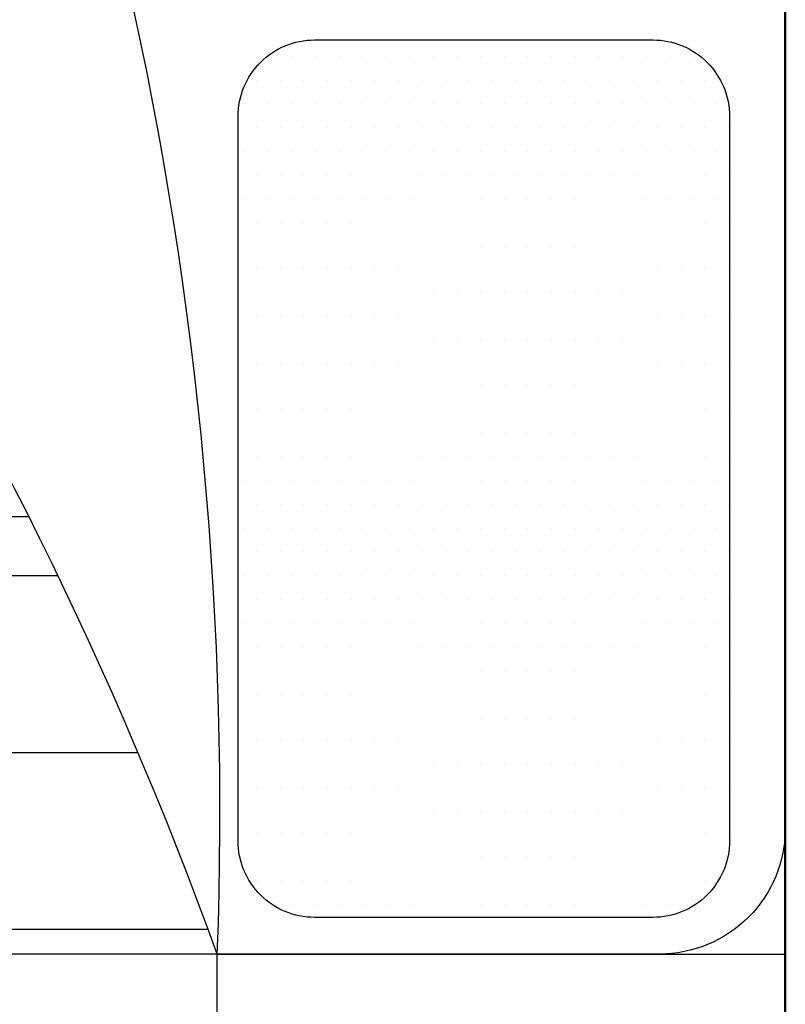
# Model space of a CAD drawing. Units: inches. Extents: x 3064 to 19385, y 846 to 15425.
# Tile 14 of 108: x 3758 to 3782, y 1032 to 1063. Entities that reach past the tile are written whole.
import ezdxf

# ---------------------------------------------------------------- set-up
doc = ezdxf.new("R2010")
doc.units = ezdxf.units.IN
doc.layers.add('A-FLOR-FIXT', color=9, linetype='Continuous', lineweight=18)
doc.layers.add('A-WALL', color=7, linetype='Continuous', lineweight=50)
doc.layers.add('BLOCK', color=6, linetype='Continuous')

# ---------------------------------------------------------------- blocks, each defined once
blk = doc.blocks.new('*X6')
at = {"color": 0}
for p, q in [((280.3125, 439.8862), (280.3125, 452.8965)), ((278.9062, 439.4824), (278.9062, 452.3385)), ((277.5, 439.4824), (277.5, 451.7019)), ((277.0312, 439.4824), (277.0312, 451.4714))]:
    blk.add_line(p, q, dxfattribs=at)
blk = doc.blocks.new('*X7')
at = {"color": 0}
for p, q in [((273.9375, 457.03125), (273.9375, 457.03125)), ((274.3125, 457.03125), (274.3125, 457.03125)), ((274.6875, 457.03125), (274.6875, 457.03125)), ((275.0625, 457.03125), (275.0625, 457.03125)), ((275.4375, 457.03125), (275.4375, 457.03125)), ((275.8125, 457.03125), (275.8125, 457.03125)), ((276.1875, 457.03125), (276.1875, 457.03125)), ((276.5625, 457.03125), (276.5625, 457.03125)), ((276.9375, 457.03125), (276.9375, 457.03125)), ((277.3125, 457.03125), (277.3125, 457.03125)), ((277.6875, 457.03125), (277.6875, 457.03125)), ((278.0625, 457.03125), (278.0625, 457.03125)), ((278.4375, 457.03125), (278.4375, 457.03125)), ((278.8125, 457.03125), (278.8125, 457.03125)), ((279.1875, 457.03125), (279.1875, 457.03125)), ((279.5625, 457.03125), (279.5625, 457.03125)), ((273.75, 456.9375), (273.75, 456.9375)), ((274.125, 456.9375), (274.125, 456.9375)), ((274.5, 456.9375), (274.5, 456.9375)), ((274.875, 456.9375), (274.875, 456.9375)), ((275.25, 456.9375), (275.25, 456.9375)), ((275.625, 456.9375), (275.625, 456.9375)), ((276, 456.9375), (276, 456.9375)), ((276.375, 456.9375), (276.375, 456.9375)), ((276.75, 456.9375), (276.75, 456.9375)), ((277.125, 456.9375), (277.125, 456.9375)), ((277.5, 456.9375), (277.5, 456.9375)), ((277.875, 456.9375), (277.875, 456.9375)), ((278.25, 456.9375), (278.25, 456.9375)), ((278.625, 456.9375), (278.625, 456.9375)), ((279, 456.9375), (279, 456.9375)), ((279.375, 456.9375), (279.375, 456.9375)), ((279.75, 456.9375), (279.75, 456.9375)), ((273.5625, 456.84375), (273.5625, 456.84375)), ((273.9375, 456.84375), (273.9375, 456.84375)), ((274.3125, 456.84375), (274.3125, 456.84375)), ((274.6875, 456.84375), (274.6875, 456.84375)), ((275.0625, 456.84375), (275.0625, 456.84375)), ((275.4375, 456.84375), (275.4375, 456.84375)), ((275.8125, 456.84375), (275.8125, 456.84375)), ((276.1875, 456.84375), (276.1875, 456.84375)), ((276.5625, 456.84375), (276.5625, 456.84375)), ((276.9375, 456.84375), (276.9375, 456.84375)), ((277.3125, 456.84375), (277.3125, 456.84375)), ((277.6875, 456.84375), (277.6875, 456.84375)), ((278.0625, 456.84375), (278.0625, 456.84375)), ((278.4375, 456.84375), (278.4375, 456.84375)), ((278.8125, 456.84375), (278.8125, 456.84375)), ((279.1875, 456.84375), (279.1875, 456.84375)), ((279.5625, 456.84375), (279.5625, 456.84375)), ((279.9375, 456.84375), (279.9375, 456.84375)), ((273.375, 456.75), (273.375, 456.75)), ((273.75, 456.75), (273.75, 456.75)), ((274.125, 456.75), (274.125, 456.75)), ((274.5, 456.75), (274.5, 456.75)), ((274.875, 456.75), (274.875, 456.75)), ((275.25, 456.75), (275.25, 456.75)), ((275.625, 456.75), (275.625, 456.75)), ((276, 456.75), (276, 456.75)), ((276.375, 456.75), (276.375, 456.75)), ((276.75, 456.75), (276.75, 456.75)), ((277.125, 456.75), (277.125, 456.75)), ((277.5, 456.75), (277.5, 456.75)), ((277.875, 456.75), (277.875, 456.75)), ((278.25, 456.75), (278.25, 456.75)), ((278.625, 456.75), (278.625, 456.75)), ((279, 456.75), (279, 456.75)), ((279.375, 456.75), (279.375, 456.75)), ((279.75, 456.75), (279.75, 456.75)), ((280.125, 456.75), (280.125, 456.75)), ((273.5625, 456.65625), (273.5625, 456.65625)), ((273.9375, 456.65625), (273.9375, 456.65625)), ((274.3125, 456.65625), (274.3125, 456.65625)), ((274.6875, 456.65625), (274.6875, 456.65625)), ((275.0625, 456.65625), (275.0625, 456.65625)), ((275.4375, 456.65625), (275.4375, 456.65625)), ((275.8125, 456.65625), (275.8125, 456.65625)), ((276.1875, 456.65625), (276.1875, 456.65625)), ((276.5625, 456.65625), (276.5625, 456.65625)), ((276.9375, 456.65625), (276.9375, 456.65625)), ((277.3125, 456.65625), (277.3125, 456.65625)), ((277.6875, 456.65625), (277.6875, 456.65625)), ((278.0625, 456.65625), (278.0625, 456.65625)), ((278.4375, 456.65625), (278.4375, 456.65625)), ((278.8125, 456.65625), (278.8125, 456.65625)), ((279.1875, 456.65625), (279.1875, 456.65625)), ((279.5625, 456.65625), (279.5625, 456.65625)), ((279.9375, 456.65625), (279.9375, 456.65625)), ((273.375, 456.5625), (273.375, 456.5625)), ((273.75, 456.5625), (273.75, 456.5625)), ((274.125, 456.5625), (274.125, 456.5625)), ((274.5, 456.5625), (274.5, 456.5625)), ((274.875, 456.5625), (274.875, 456.5625)), ((275.25, 456.5625), (275.25, 456.5625)), ((275.625, 456.5625), (275.625, 456.5625)), ((276, 456.5625), (276, 456.5625)), ((276.375, 456.5625), (276.375, 456.5625)), ((276.75, 456.5625), (276.75, 456.5625)), ((277.125, 456.5625), (277.125, 456.5625)), ((277.5, 456.5625), (277.5, 456.5625)), ((277.875, 456.5625), (277.875, 456.5625)), ((278.25, 456.5625), (278.25, 456.5625)), ((278.625, 456.5625), (278.625, 456.5625)), ((279, 456.5625), (279, 456.5625)), ((279.375, 456.5625), (279.375, 456.5625)), ((279.75, 456.5625), (279.75, 456.5625)), ((280.125, 456.5625), (280.125, 456.5625)), ((273.5625, 456.46875), (273.5625, 456.46875)), ((273.9375, 456.46875), (273.9375, 456.46875)), ((274.3125, 456.46875), (274.3125, 456.46875)), ((274.6875, 456.46875), (274.6875, 456.46875)), ((275.0625, 456.46875), (275.0625, 456.46875)), ((275.4375, 456.46875), (275.4375, 456.46875)), ((275.8125, 456.46875), (275.8125, 456.46875)), ((276.1875, 456.46875), (276.1875, 456.46875)), ((276.5625, 456.46875), (276.5625, 456.46875)), ((276.9375, 456.46875), (276.9375, 456.46875)), ((277.3125, 456.46875), (277.3125, 456.46875)), ((277.6875, 456.46875), (277.6875, 456.46875)), ((278.0625, 456.46875), (278.0625, 456.46875)), ((278.4375, 456.46875), (278.4375, 456.46875)), ((278.8125, 456.46875), (278.8125, 456.46875)), ((279.1875, 456.46875), (279.1875, 456.46875)), ((279.5625, 456.46875), (279.5625, 456.46875)), ((279.9375, 456.46875), (279.9375, 456.46875)), ((273.375, 456.375), (273.375, 456.375)), ((273.75, 456.375), (273.75, 456.375)), ((274.125, 456.375), (274.125, 456.375)), ((274.5, 456.375), (274.5, 456.375)), ((274.875, 456.375), (274.875, 456.375)), ((275.25, 456.375), (275.25, 456.375)), ((275.625, 456.375), (275.625, 456.375)), ((276, 456.375), (276, 456.375)), ((276.375, 456.375), (276.375, 456.375)), ((276.75, 456.375), (276.75, 456.375)), ((277.125, 456.375), (277.125, 456.375)), ((277.5, 456.375), (277.5, 456.375)), ((277.875, 456.375), (277.875, 456.375)), ((278.25, 456.375), (278.25, 456.375)), ((278.625, 456.375), (278.625, 456.375)), ((279, 456.375), (279, 456.375)), ((279.375, 456.375), (279.375, 456.375)), ((279.75, 456.375), (279.75, 456.375)), ((280.125, 456.375), (280.125, 456.375)), ((273.5625, 456.28125), (273.5625, 456.28125)), ((273.9375, 456.28125), (273.9375, 456.28125)), ((274.3125, 456.28125), (274.3125, 456.28125)), ((274.6875, 456.28125), (274.6875, 456.28125)), ((275.0625, 456.28125), (275.0625, 456.28125)), ((275.4375, 456.28125), (275.4375, 456.28125)), ((275.8125, 456.28125), (275.8125, 456.28125)), ((276.1875, 456.28125), (276.1875, 456.28125)), ((276.5625, 456.28125), (276.5625, 456.28125)), ((276.9375, 456.28125), (276.9375, 456.28125)), ((277.3125, 456.28125), (277.3125, 456.28125)), ((277.6875, 456.28125), (277.6875, 456.28125)), ((278.0625, 456.28125), (278.0625, 456.28125)), ((278.4375, 456.28125), (278.4375, 456.28125)), ((278.8125, 456.28125), (278.8125, 456.28125)), ((279.1875, 456.28125), (279.1875, 456.28125)), ((279.5625, 456.28125), (279.5625, 456.28125)), ((279.9375, 456.28125), (279.9375, 456.28125)), ((273.375, 456.1875), (273.375, 456.1875)), ((273.75, 456.1875), (273.75, 456.1875)), ((274.125, 456.1875), (274.125, 456.1875)), ((274.5, 456.1875), (274.5, 456.1875)), ((274.875, 456.1875), (274.875, 456.1875)), ((275.25, 456.1875), (275.25, 456.1875)), ((275.625, 456.1875), (275.625, 456.1875)), ((276, 456.1875), (276, 456.1875)), ((276.375, 456.1875), (276.375, 456.1875)), ((276.75, 456.1875), (276.75, 456.1875)), ((277.125, 456.1875), (277.125, 456.1875)), ((277.5, 456.1875), (277.5, 456.1875)), ((277.875, 456.1875), (277.875, 456.1875)), ((278.25, 456.1875), (278.25, 456.1875)), ((278.625, 456.1875), (278.625, 456.1875)), ((279, 456.1875), (279, 456.1875)), ((279.375, 456.1875), (279.375, 456.1875)), ((279.75, 456.1875), (279.75, 456.1875)), ((280.125, 456.1875), (280.125, 456.1875)), ((273.5625, 456.09375), (273.5625, 456.09375)), ((273.9375, 456.09375), (273.9375, 456.09375)), ((274.3125, 456.09375), (274.3125, 456.09375)), ((274.6875, 456.09375), (274.6875, 456.09375)), ((275.0625, 456.09375), (275.0625, 456.09375)), ((275.4375, 456.09375), (275.4375, 456.09375)), ((275.8125, 456.09375), (275.8125, 456.09375)), ((276.1875, 456.09375), (276.1875, 456.09375)), ((276.5625, 456.09375), (276.5625, 456.09375)), ((276.9375, 456.09375), (276.9375, 456.09375)), ((277.3125, 456.09375), (277.3125, 456.09375)), ((277.6875, 456.09375), (277.6875, 456.09375)), ((278.0625, 456.09375), (278.0625, 456.09375)), ((278.4375, 456.09375), (278.4375, 456.09375)), ((278.8125, 456.09375), (278.8125, 456.09375)), ((279.1875, 456.09375), (279.1875, 456.09375)), ((279.5625, 456.09375), (279.5625, 456.09375)), ((279.9375, 456.09375), (279.9375, 456.09375)), ((273.375, 456), (273.375, 456)), ((273.75, 456), (273.75, 456)), ((274.125, 456), (274.125, 456)), ((274.5, 456), (274.5, 456)), ((274.875, 456), (274.875, 456)), ((275.25, 456), (275.25, 456)), ((275.625, 456), (275.625, 456)), ((276, 456), (276, 456)), ((276.375, 456), (276.375, 456)), ((276.75, 456), (276.75, 456)), ((277.125, 456), (277.125, 456)), ((277.5, 456), (277.5, 456)), ((277.875, 456), (277.875, 456)), ((278.25, 456), (278.25, 456)), ((278.625, 456), (278.625, 456)), ((279, 456), (279, 456)), ((279.375, 456), (279.375, 456)), ((279.75, 456), (279.75, 456)), ((280.125, 456), (280.125, 456)), ((273.5625, 455.90625), (273.5625, 455.90625)), ((273.9375, 455.90625), (273.9375, 455.90625)), ((274.3125, 455.90625), (274.3125, 455.90625)), ((274.6875, 455.90625), (274.6875, 455.90625)), ((275.0625, 455.90625), (275.0625, 455.90625)), ((275.4375, 455.90625), (275.4375, 455.90625)), ((275.8125, 455.90625), (275.8125, 455.90625)), ((276.1875, 455.90625), (276.1875, 455.90625)), ((276.5625, 455.90625), (276.5625, 455.90625)), ((276.9375, 455.90625), (276.9375, 455.90625)), ((277.3125, 455.90625), (277.3125, 455.90625)), ((277.6875, 455.90625), (277.6875, 455.90625)), ((278.0625, 455.90625), (278.0625, 455.90625)), ((278.4375, 455.90625), (278.4375, 455.90625)), ((278.8125, 455.90625), (278.8125, 455.90625)), ((279.1875, 455.90625), (279.1875, 455.90625)), ((279.5625, 455.90625), (279.5625, 455.90625)), ((279.9375, 455.90625), (279.9375, 455.90625)), ((273.375, 455.8125), (273.375, 455.8125)), ((273.75, 455.8125), (273.75, 455.8125)), ((274.125, 455.8125), (274.125, 455.8125)), ((274.5, 455.8125), (274.5, 455.8125)), ((274.875, 455.8125), (274.875, 455.8125)), ((275.25, 455.8125), (275.25, 455.8125)), ((275.625, 455.8125), (275.625, 455.8125)), ((276, 455.8125), (276, 455.8125)), ((276.375, 455.8125), (276.375, 455.8125)), ((276.75, 455.8125), (276.75, 455.8125)), ((277.125, 455.8125), (277.125, 455.8125)), ((277.5, 455.8125), (277.5, 455.8125)), ((277.875, 455.8125), (277.875, 455.8125)), ((278.25, 455.8125), (278.25, 455.8125)), ((278.625, 455.8125), (278.625, 455.8125)), ((279, 455.8125), (279, 455.8125)), ((279.375, 455.8125), (279.375, 455.8125)), ((279.75, 455.8125), (279.75, 455.8125)), ((280.125, 455.8125), (280.125, 455.8125)), ((273.5625, 455.71875), (273.5625, 455.71875)), ((273.9375, 455.71875), (273.9375, 455.71875)), ((274.3125, 455.71875), (274.3125, 455.71875)), ((274.6875, 455.71875), (274.6875, 455.71875)), ((275.0625, 455.71875), (275.0625, 455.71875)), ((275.4375, 455.71875), (275.4375, 455.71875)), ((275.8125, 455.71875), (275.8125, 455.71875)), ((276.1875, 455.71875), (276.1875, 455.71875)), ((276.5625, 455.71875), (276.5625, 455.71875)), ((276.9375, 455.71875), (276.9375, 455.71875)), ((277.3125, 455.71875), (277.3125, 455.71875)), ((277.6875, 455.71875), (277.6875, 455.71875)), ((278.0625, 455.71875), (278.0625, 455.71875)), ((278.4375, 455.71875), (278.4375, 455.71875)), ((278.8125, 455.71875), (278.8125, 455.71875)), ((279.1875, 455.71875), (279.1875, 455.71875)), ((279.5625, 455.71875), (279.5625, 455.71875)), ((279.9375, 455.71875), (279.9375, 455.71875)), ((273.375, 455.625), (273.375, 455.625)), ((273.75, 455.625), (273.75, 455.625)), ((274.125, 455.625), (274.125, 455.625)), ((274.5, 455.625), (274.5, 455.625)), ((274.875, 455.625), (274.875, 455.625)), ((275.25, 455.625), (275.25, 455.625)), ((275.625, 455.625), (275.625, 455.625)), ((276, 455.625), (276, 455.625)), ((276.375, 455.625), (276.375, 455.625)), ((276.75, 455.625), (276.75, 455.625)), ((277.125, 455.625), (277.125, 455.625)), ((277.5, 455.625), (277.5, 455.625)), ((277.875, 455.625), (277.875, 455.625)), ((278.25, 455.625), (278.25, 455.625)), ((278.625, 455.625), (278.625, 455.625)), ((279, 455.625), (279, 455.625)), ((279.375, 455.625), (279.375, 455.625)), ((279.75, 455.625), (279.75, 455.625)), ((280.125, 455.625), (280.125, 455.625)), ((273.5625, 455.53125), (273.5625, 455.53125)), ((273.9375, 455.53125), (273.9375, 455.53125)), ((274.3125, 455.53125), (274.3125, 455.53125)), ((274.6875, 455.53125), (274.6875, 455.53125)), ((275.0625, 455.53125), (275.0625, 455.53125)), ((275.4375, 455.53125), (275.4375, 455.53125)), ((275.8125, 455.53125), (275.8125, 455.53125)), ((276.1875, 455.53125), (276.1875, 455.53125)), ((276.5625, 455.53125), (276.5625, 455.53125)), ((276.9375, 455.53125), (276.9375, 455.53125)), ((277.3125, 455.53125), (277.3125, 455.53125)), ((277.6875, 455.53125), (277.6875, 455.53125)), ((278.0625, 455.53125), (278.0625, 455.53125)), ((278.4375, 455.53125), (278.4375, 455.53125)), ((278.8125, 455.53125), (278.8125, 455.53125)), ((279.1875, 455.53125), (279.1875, 455.53125)), ((279.5625, 455.53125), (279.5625, 455.53125)), ((279.9375, 455.53125), (279.9375, 455.53125)), ((273.375, 455.4375), (273.375, 455.4375)), ((273.75, 455.4375), (273.75, 455.4375)), ((274.125, 455.4375), (274.125, 455.4375)), ((274.5, 455.4375), (274.5, 455.4375)), ((274.875, 455.4375), (274.875, 455.4375)), ((275.25, 455.4375), (275.25, 455.4375)), ((275.625, 455.4375), (275.625, 455.4375)), ((276, 455.4375), (276, 455.4375)), ((276.375, 455.4375), (276.375, 455.4375)), ((276.75, 455.4375), (276.75, 455.4375)), ((277.125, 455.4375), (277.125, 455.4375)), ((277.5, 455.4375), (277.5, 455.4375)), ((277.875, 455.4375), (277.875, 455.4375)), ((278.25, 455.4375), (278.25, 455.4375)), ((278.625, 455.4375), (278.625, 455.4375)), ((279, 455.4375), (279, 455.4375)), ((279.375, 455.4375), (279.375, 455.4375)), ((279.75, 455.4375), (279.75, 455.4375)), ((280.125, 455.4375), (280.125, 455.4375)), ((273.5625, 455.34375), (273.5625, 455.34375)), ((273.9375, 455.34375), (273.9375, 455.34375)), ((274.3125, 455.34375), (274.3125, 455.34375)), ((274.6875, 455.34375), (274.6875, 455.34375)), ((275.0625, 455.34375), (275.0625, 455.34375)), ((275.4375, 455.34375), (275.4375, 455.34375)), ((275.8125, 455.34375), (275.8125, 455.34375)), ((276.1875, 455.34375), (276.1875, 455.34375)), ((276.5625, 455.34375), (276.5625, 455.34375)), ((276.9375, 455.34375), (276.9375, 455.34375)), ((277.3125, 455.34375), (277.3125, 455.34375)), ((277.6875, 455.34375), (277.6875, 455.34375)), ((278.0625, 455.34375), (278.0625, 455.34375)), ((278.4375, 455.34375), (278.4375, 455.34375)), ((278.8125, 455.34375), (278.8125, 455.34375)), ((279.1875, 455.34375), (279.1875, 455.34375)), ((279.5625, 455.34375), (279.5625, 455.34375)), ((279.9375, 455.34375), (279.9375, 455.34375)), ((273.375, 455.25), (273.375, 455.25)), ((273.75, 455.25), (273.75, 455.25)), ((274.125, 455.25), (274.125, 455.25)), ((274.5, 455.25), (274.5, 455.25)), ((274.875, 455.25), (274.875, 455.25)), ((275.25, 455.25), (275.25, 455.25)), ((275.625, 455.25), (275.625, 455.25)), ((276, 455.25), (276, 455.25)), ((276.375, 455.25), (276.375, 455.25)), ((276.75, 455.25), (276.75, 455.25)), ((277.125, 455.25), (277.125, 455.25)), ((277.5, 455.25), (277.5, 455.25)), ((277.875, 455.25), (277.875, 455.25)), ((278.25, 455.25), (278.25, 455.25)), ((278.625, 455.25), (278.625, 455.25)), ((279, 455.25), (279, 455.25)), ((279.375, 455.25), (279.375, 455.25)), ((279.75, 455.25), (279.75, 455.25)), ((280.125, 455.25), (280.125, 455.25)), ((273.5625, 455.15625), (273.5625, 455.15625)), ((273.9375, 455.15625), (273.9375, 455.15625)), ((274.3125, 455.15625), (274.3125, 455.15625)), ((274.6875, 455.15625), (274.6875, 455.15625)), ((275.0625, 455.15625), (275.0625, 455.15625)), ((275.4375, 455.15625), (275.4375, 455.15625)), ((275.8125, 455.15625), (275.8125, 455.15625)), ((276.1875, 455.15625), (276.1875, 455.15625)), ((276.5625, 455.15625), (276.5625, 455.15625)), ((276.9375, 455.15625), (276.9375, 455.15625)), ((277.3125, 455.15625), (277.3125, 455.15625)), ((277.6875, 455.15625), (277.6875, 455.15625)), ((278.0625, 455.15625), (278.0625, 455.15625)), ((278.4375, 455.15625), (278.4375, 455.15625)), ((278.8125, 455.15625), (278.8125, 455.15625)), ((279.1875, 455.15625), (279.1875, 455.15625)), ((279.5625, 455.15625), (279.5625, 455.15625)), ((279.9375, 455.15625), (279.9375, 455.15625)), ((273.375, 455.0625), (273.375, 455.0625)), ((273.75, 455.0625), (273.75, 455.0625)), ((274.125, 455.0625), (274.125, 455.0625)), ((274.5, 455.0625), (274.5, 455.0625)), ((274.875, 455.0625), (274.875, 455.0625)), ((275.25, 455.0625), (275.25, 455.0625)), ((275.625, 455.0625), (275.625, 455.0625)), ((276, 455.0625), (276, 455.0625)), ((276.375, 455.0625), (276.375, 455.0625)), ((276.75, 455.0625), (276.75, 455.0625)), ((277.125, 455.0625), (277.125, 455.0625)), ((277.5, 455.0625), (277.5, 455.0625)), ((277.875, 455.0625), (277.875, 455.0625)), ((278.25, 455.0625), (278.25, 455.0625)), ((278.625, 455.0625), (278.625, 455.0625)), ((279, 455.0625), (279, 455.0625)), ((279.375, 455.0625), (279.375, 455.0625)), ((279.75, 455.0625), (279.75, 455.0625)), ((280.125, 455.0625), (280.125, 455.0625)), ((273.5625, 454.96875), (273.5625, 454.96875)), ((273.9375, 454.96875), (273.9375, 454.96875)), ((274.3125, 454.96875), (274.3125, 454.96875)), ((274.6875, 454.96875), (274.6875, 454.96875)), ((275.0625, 454.96875), (275.0625, 454.96875)), ((275.4375, 454.96875), (275.4375, 454.96875)), ((275.8125, 454.96875), (275.8125, 454.96875)), ((276.1875, 454.96875), (276.1875, 454.96875)), ((276.5625, 454.96875), (276.5625, 454.96875)), ((276.9375, 454.96875), (276.9375, 454.96875)), ((277.3125, 454.96875), (277.3125, 454.96875)), ((277.6875, 454.96875), (277.6875, 454.96875)), ((278.0625, 454.96875), (278.0625, 454.96875)), ((278.4375, 454.96875), (278.4375, 454.96875)), ((278.8125, 454.96875), (278.8125, 454.96875)), ((279.1875, 454.96875), (279.1875, 454.96875)), ((279.5625, 454.96875), (279.5625, 454.96875)), ((279.9375, 454.96875), (279.9375, 454.96875)), ((273.375, 454.875), (273.375, 454.875)), ((273.75, 454.875), (273.75, 454.875)), ((274.125, 454.875), (274.125, 454.875)), ((274.5, 454.875), (274.5, 454.875)), ((274.875, 454.875), (274.875, 454.875)), ((275.25, 454.875), (275.25, 454.875)), ((275.625, 454.875), (275.625, 454.875)), ((276, 454.875), (276, 454.875)), ((276.375, 454.875), (276.375, 454.875)), ((276.75, 454.875), (276.75, 454.875)), ((277.125, 454.875), (277.125, 454.875)), ((277.5, 454.875), (277.5, 454.875)), ((277.875, 454.875), (277.875, 454.875)), ((278.25, 454.875), (278.25, 454.875)), ((278.625, 454.875), (278.625, 454.875)), ((279, 454.875), (279, 454.875)), ((279.375, 454.875), (279.375, 454.875)), ((279.75, 454.875), (279.75, 454.875)), ((280.125, 454.875), (280.125, 454.875)), ((273.5625, 454.78125), (273.5625, 454.78125)), ((273.9375, 454.78125), (273.9375, 454.78125)), ((274.3125, 454.78125), (274.3125, 454.78125)), ((274.6875, 454.78125), (274.6875, 454.78125)), ((275.0625, 454.78125), (275.0625, 454.78125)), ((275.4375, 454.78125), (275.4375, 454.78125)), ((275.8125, 454.78125), (275.8125, 454.78125)), ((276.1875, 454.78125), (276.1875, 454.78125)), ((276.5625, 454.78125), (276.5625, 454.78125)), ((276.9375, 454.78125), (276.9375, 454.78125)), ((277.3125, 454.78125), (277.3125, 454.78125)), ((277.6875, 454.78125), (277.6875, 454.78125)), ((278.0625, 454.78125), (278.0625, 454.78125)), ((278.4375, 454.78125), (278.4375, 454.78125)), ((278.8125, 454.78125), (278.8125, 454.78125)), ((279.1875, 454.78125), (279.1875, 454.78125)), ((279.5625, 454.78125), (279.5625, 454.78125)), ((279.9375, 454.78125), (279.9375, 454.78125)), ((273.375, 454.6875), (273.375, 454.6875)), ((273.75, 454.6875), (273.75, 454.6875)), ((274.125, 454.6875), (274.125, 454.6875)), ((274.5, 454.6875), (274.5, 454.6875)), ((274.875, 454.6875), (274.875, 454.6875)), ((275.25, 454.6875), (275.25, 454.6875)), ((275.625, 454.6875), (275.625, 454.6875)), ((276, 454.6875), (276, 454.6875)), ((276.375, 454.6875), (276.375, 454.6875)), ((276.75, 454.6875), (276.75, 454.6875)), ((277.125, 454.6875), (277.125, 454.6875)), ((277.5, 454.6875), (277.5, 454.6875)), ((277.875, 454.6875), (277.875, 454.6875)), ((278.25, 454.6875), (278.25, 454.6875)), ((278.625, 454.6875), (278.625, 454.6875)), ((279, 454.6875), (279, 454.6875)), ((279.375, 454.6875), (279.375, 454.6875)), ((279.75, 454.6875), (279.75, 454.6875)), ((280.125, 454.6875), (280.125, 454.6875)), ((273.5625, 454.59375), (273.5625, 454.59375)), ((273.9375, 454.59375), (273.9375, 454.59375)), ((274.3125, 454.59375), (274.3125, 454.59375)), ((274.6875, 454.59375), (274.6875, 454.59375)), ((275.0625, 454.59375), (275.0625, 454.59375)), ((275.4375, 454.59375), (275.4375, 454.59375)), ((275.8125, 454.59375), (275.8125, 454.59375)), ((276.1875, 454.59375), (276.1875, 454.59375)), ((276.5625, 454.59375), (276.5625, 454.59375)), ((276.9375, 454.59375), (276.9375, 454.59375)), ((277.3125, 454.59375), (277.3125, 454.59375)), ((277.6875, 454.59375), (277.6875, 454.59375)), ((278.0625, 454.59375), (278.0625, 454.59375)), ((278.4375, 454.59375), (278.4375, 454.59375)), ((278.8125, 454.59375), (278.8125, 454.59375)), ((279.1875, 454.59375), (279.1875, 454.59375)), ((279.5625, 454.59375), (279.5625, 454.59375)), ((279.9375, 454.59375), (279.9375, 454.59375)), ((273.375, 454.5), (273.375, 454.5)), ((273.75, 454.5), (273.75, 454.5)), ((274.125, 454.5), (274.125, 454.5)), ((274.5, 454.5), (274.5, 454.5)), ((274.875, 454.5), (274.875, 454.5)), ((275.25, 454.5), (275.25, 454.5)), ((275.625, 454.5), (275.625, 454.5)), ((276, 454.5), (276, 454.5)), ((276.375, 454.5), (276.375, 454.5)), ((276.75, 454.5), (276.75, 454.5)), ((277.125, 454.5), (277.125, 454.5)), ((277.5, 454.5), (277.5, 454.5)), ((277.875, 454.5), (277.875, 454.5)), ((278.25, 454.5), (278.25, 454.5)), ((278.625, 454.5), (278.625, 454.5)), ((279, 454.5), (279, 454.5)), ((279.375, 454.5), (279.375, 454.5)), ((279.75, 454.5), (279.75, 454.5)), ((280.125, 454.5), (280.125, 454.5)), ((273.5625, 454.40625), (273.5625, 454.40625)), ((273.9375, 454.40625), (273.9375, 454.40625)), ((274.3125, 454.40625), (274.3125, 454.40625)), ((274.6875, 454.40625), (274.6875, 454.40625)), ((275.0625, 454.40625), (275.0625, 454.40625)), ((275.4375, 454.40625), (275.4375, 454.40625)), ((275.8125, 454.40625), (275.8125, 454.40625)), ((276.1875, 454.40625), (276.1875, 454.40625)), ((276.5625, 454.40625), (276.5625, 454.40625)), ((276.9375, 454.40625), (276.9375, 454.40625)), ((277.3125, 454.40625), (277.3125, 454.40625)), ((277.6875, 454.40625), (277.6875, 454.40625)), ((278.0625, 454.40625), (278.0625, 454.40625)), ((278.4375, 454.40625), (278.4375, 454.40625)), ((278.8125, 454.40625), (278.8125, 454.40625)), ((279.1875, 454.40625), (279.1875, 454.40625)), ((279.5625, 454.40625), (279.5625, 454.40625)), ((279.9375, 454.40625), (279.9375, 454.40625)), ((273.375, 454.3125), (273.375, 454.3125)), ((273.75, 454.3125), (273.75, 454.3125)), ((274.125, 454.3125), (274.125, 454.3125)), ((274.5, 454.3125), (274.5, 454.3125)), ((274.875, 454.3125), (274.875, 454.3125)), ((275.25, 454.3125), (275.25, 454.3125)), ((275.625, 454.3125), (275.625, 454.3125)), ((276, 454.3125), (276, 454.3125)), ((276.375, 454.3125), (276.375, 454.3125)), ((276.75, 454.3125), (276.75, 454.3125)), ((277.125, 454.3125), (277.125, 454.3125)), ((277.5, 454.3125), (277.5, 454.3125)), ((277.875, 454.3125), (277.875, 454.3125)), ((278.25, 454.3125), (278.25, 454.3125)), ((278.625, 454.3125), (278.625, 454.3125)), ((279, 454.3125), (279, 454.3125)), ((279.375, 454.3125), (279.375, 454.3125)), ((279.75, 454.3125), (279.75, 454.3125)), ((280.125, 454.3125), (280.125, 454.3125)), ((273.5625, 454.21875), (273.5625, 454.21875)), ((273.9375, 454.21875), (273.9375, 454.21875)), ((274.3125, 454.21875), (274.3125, 454.21875)), ((274.6875, 454.21875), (274.6875, 454.21875)), ((275.0625, 454.21875), (275.0625, 454.21875)), ((275.4375, 454.21875), (275.4375, 454.21875)), ((275.8125, 454.21875), (275.8125, 454.21875)), ((276.1875, 454.21875), (276.1875, 454.21875)), ((276.5625, 454.21875), (276.5625, 454.21875)), ((276.9375, 454.21875), (276.9375, 454.21875)), ((277.3125, 454.21875), (277.3125, 454.21875)), ((277.6875, 454.21875), (277.6875, 454.21875)), ((278.0625, 454.21875), (278.0625, 454.21875)), ((278.4375, 454.21875), (278.4375, 454.21875)), ((278.8125, 454.21875), (278.8125, 454.21875)), ((279.1875, 454.21875), (279.1875, 454.21875)), ((279.5625, 454.21875), (279.5625, 454.21875)), ((279.9375, 454.21875), (279.9375, 454.21875)), ((273.375, 454.125), (273.375, 454.125)), ((273.75, 454.125), (273.75, 454.125)), ((274.125, 454.125), (274.125, 454.125)), ((274.5, 454.125), (274.5, 454.125)), ((274.875, 454.125), (274.875, 454.125)), ((275.25, 454.125), (275.25, 454.125)), ((275.625, 454.125), (275.625, 454.125)), ((276, 454.125), (276, 454.125)), ((276.375, 454.125), (276.375, 454.125)), ((276.75, 454.125), (276.75, 454.125)), ((277.125, 454.125), (277.125, 454.125)), ((277.5, 454.125), (277.5, 454.125)), ((277.875, 454.125), (277.875, 454.125)), ((278.25, 454.125), (278.25, 454.125)), ((278.625, 454.125), (278.625, 454.125)), ((279, 454.125), (279, 454.125)), ((279.375, 454.125), (279.375, 454.125)), ((279.75, 454.125), (279.75, 454.125)), ((280.125, 454.125), (280.125, 454.125)), ((273.5625, 454.03125), (273.5625, 454.03125)), ((273.9375, 454.03125), (273.9375, 454.03125)), ((274.3125, 454.03125), (274.3125, 454.03125)), ((274.6875, 454.03125), (274.6875, 454.03125)), ((275.0625, 454.03125), (275.0625, 454.03125)), ((275.4375, 454.03125), (275.4375, 454.03125)), ((275.8125, 454.03125), (275.8125, 454.03125)), ((276.1875, 454.03125), (276.1875, 454.03125)), ((276.5625, 454.03125), (276.5625, 454.03125)), ((276.9375, 454.03125), (276.9375, 454.03125)), ((277.3125, 454.03125), (277.3125, 454.03125)), ((277.6875, 454.03125), (277.6875, 454.03125)), ((278.0625, 454.03125), (278.0625, 454.03125)), ((278.4375, 454.03125), (278.4375, 454.03125)), ((278.8125, 454.03125), (278.8125, 454.03125)), ((279.1875, 454.03125), (279.1875, 454.03125)), ((279.5625, 454.03125), (279.5625, 454.03125)), ((279.9375, 454.03125), (279.9375, 454.03125)), ((273.375, 453.9375), (273.375, 453.9375)), ((273.75, 453.9375), (273.75, 453.9375)), ((274.125, 453.9375), (274.125, 453.9375)), ((274.5, 453.9375), (274.5, 453.9375)), ((274.875, 453.9375), (274.875, 453.9375)), ((275.25, 453.9375), (275.25, 453.9375)), ((275.625, 453.9375), (275.625, 453.9375)), ((276, 453.9375), (276, 453.9375)), ((276.375, 453.9375), (276.375, 453.9375)), ((276.75, 453.9375), (276.75, 453.9375)), ((277.125, 453.9375), (277.125, 453.9375)), ((277.5, 453.9375), (277.5, 453.9375)), ((277.875, 453.9375), (277.875, 453.9375)), ((278.25, 453.9375), (278.25, 453.9375)), ((278.625, 453.9375), (278.625, 453.9375)), ((279, 453.9375), (279, 453.9375)), ((279.375, 453.9375), (279.375, 453.9375)), ((279.75, 453.9375), (279.75, 453.9375)), ((280.125, 453.9375), (280.125, 453.9375)), ((273.5625, 453.84375), (273.5625, 453.84375)), ((273.9375, 453.84375), (273.9375, 453.84375)), ((274.3125, 453.84375), (274.3125, 453.84375)), ((274.6875, 453.84375), (274.6875, 453.84375)), ((275.0625, 453.84375), (275.0625, 453.84375)), ((275.4375, 453.84375), (275.4375, 453.84375)), ((275.8125, 453.84375), (275.8125, 453.84375)), ((276.1875, 453.84375), (276.1875, 453.84375)), ((276.5625, 453.84375), (276.5625, 453.84375)), ((276.9375, 453.84375), (276.9375, 453.84375)), ((277.3125, 453.84375), (277.3125, 453.84375)), ((277.6875, 453.84375), (277.6875, 453.84375)), ((278.0625, 453.84375), (278.0625, 453.84375)), ((278.4375, 453.84375), (278.4375, 453.84375)), ((278.8125, 453.84375), (278.8125, 453.84375)), ((279.1875, 453.84375), (279.1875, 453.84375)), ((279.5625, 453.84375), (279.5625, 453.84375)), ((279.9375, 453.84375), (279.9375, 453.84375)), ((273.375, 453.75), (273.375, 453.75)), ((273.75, 453.75), (273.75, 453.75)), ((274.125, 453.75), (274.125, 453.75)), ((274.5, 453.75), (274.5, 453.75)), ((274.875, 453.75), (274.875, 453.75)), ((275.25, 453.75), (275.25, 453.75)), ((275.625, 453.75), (275.625, 453.75)), ((276, 453.75), (276, 453.75)), ((276.375, 453.75), (276.375, 453.75)), ((276.75, 453.75), (276.75, 453.75)), ((277.125, 453.75), (277.125, 453.75)), ((277.5, 453.75), (277.5, 453.75)), ((277.875, 453.75), (277.875, 453.75)), ((278.25, 453.75), (278.25, 453.75)), ((278.625, 453.75), (278.625, 453.75)), ((279, 453.75), (279, 453.75)), ((279.375, 453.75), (279.375, 453.75)), ((279.75, 453.75), (279.75, 453.75)), ((280.125, 453.75), (280.125, 453.75)), ((273.5625, 453.65625), (273.5625, 453.65625)), ((273.9375, 453.65625), (273.9375, 453.65625)), ((274.3125, 453.65625), (274.3125, 453.65625)), ((274.6875, 453.65625), (274.6875, 453.65625)), ((275.0625, 453.65625), (275.0625, 453.65625)), ((275.4375, 453.65625), (275.4375, 453.65625)), ((275.8125, 453.65625), (275.8125, 453.65625)), ((276.1875, 453.65625), (276.1875, 453.65625)), ((276.5625, 453.65625), (276.5625, 453.65625)), ((276.9375, 453.65625), (276.9375, 453.65625)), ((277.3125, 453.65625), (277.3125, 453.65625)), ((277.6875, 453.65625), (277.6875, 453.65625)), ((278.0625, 453.65625), (278.0625, 453.65625)), ((278.4375, 453.65625), (278.4375, 453.65625)), ((278.8125, 453.65625), (278.8125, 453.65625)), ((279.1875, 453.65625), (279.1875, 453.65625)), ((279.5625, 453.65625), (279.5625, 453.65625)), ((279.9375, 453.65625), (279.9375, 453.65625)), ((273.375, 453.5625), (273.375, 453.5625)), ((273.75, 453.5625), (273.75, 453.5625)), ((274.125, 453.5625), (274.125, 453.5625)), ((274.5, 453.5625), (274.5, 453.5625)), ((274.875, 453.5625), (274.875, 453.5625)), ((275.25, 453.5625), (275.25, 453.5625)), ((275.625, 453.5625), (275.625, 453.5625)), ((276, 453.5625), (276, 453.5625)), ((276.375, 453.5625), (276.375, 453.5625)), ((276.75, 453.5625), (276.75, 453.5625)), ((277.125, 453.5625), (277.125, 453.5625)), ((277.5, 453.5625), (277.5, 453.5625)), ((277.875, 453.5625), (277.875, 453.5625)), ((278.25, 453.5625), (278.25, 453.5625)), ((278.625, 453.5625), (278.625, 453.5625)), ((279, 453.5625), (279, 453.5625)), ((279.375, 453.5625), (279.375, 453.5625)), ((279.75, 453.5625), (279.75, 453.5625)), ((280.125, 453.5625), (280.125, 453.5625)), ((273.5625, 453.46875), (273.5625, 453.46875)), ((273.9375, 453.46875), (273.9375, 453.46875)), ((274.3125, 453.46875), (274.3125, 453.46875)), ((274.6875, 453.46875), (274.6875, 453.46875)), ((275.0625, 453.46875), (275.0625, 453.46875)), ((275.4375, 453.46875), (275.4375, 453.46875)), ((275.8125, 453.46875), (275.8125, 453.46875)), ((276.1875, 453.46875), (276.1875, 453.46875)), ((276.5625, 453.46875), (276.5625, 453.46875)), ((276.9375, 453.46875), (276.9375, 453.46875)), ((277.3125, 453.46875), (277.3125, 453.46875)), ((277.6875, 453.46875), (277.6875, 453.46875)), ((278.0625, 453.46875), (278.0625, 453.46875)), ((278.4375, 453.46875), (278.4375, 453.46875)), ((278.8125, 453.46875), (278.8125, 453.46875)), ((279.1875, 453.46875), (279.1875, 453.46875)), ((279.5625, 453.46875), (279.5625, 453.46875)), ((279.9375, 453.46875), (279.9375, 453.46875)), ((273.375, 453.375), (273.375, 453.375)), ((273.75, 453.375), (273.75, 453.375)), ((274.125, 453.375), (274.125, 453.375)), ((274.5, 453.375), (274.5, 453.375)), ((274.875, 453.375), (274.875, 453.375)), ((275.25, 453.375), (275.25, 453.375)), ((275.625, 453.375), (275.625, 453.375)), ((276, 453.375), (276, 453.375)), ((276.375, 453.375), (276.375, 453.375)), ((276.75, 453.375), (276.75, 453.375)), ((277.125, 453.375), (277.125, 453.375)), ((277.5, 453.375), (277.5, 453.375)), ((277.875, 453.375), (277.875, 453.375)), ((278.25, 453.375), (278.25, 453.375)), ((278.625, 453.375), (278.625, 453.375)), ((279, 453.375), (279, 453.375)), ((279.375, 453.375), (279.375, 453.375)), ((279.75, 453.375), (279.75, 453.375)), ((273.5625, 453.28125), (273.5625, 453.28125)), ((273.9375, 453.28125), (273.9375, 453.28125)), ((274.3125, 453.28125), (274.3125, 453.28125)), ((274.6875, 453.28125), (274.6875, 453.28125)), ((275.0625, 453.28125), (275.0625, 453.28125)), ((275.4375, 453.28125), (275.4375, 453.28125)), ((275.8125, 453.28125), (275.8125, 453.28125)), ((276.1875, 453.28125), (276.1875, 453.28125)), ((276.5625, 453.28125), (276.5625, 453.28125)), ((276.9375, 453.28125), (276.9375, 453.28125)), ((277.3125, 453.28125), (277.3125, 453.28125)), ((277.6875, 453.28125), (277.6875, 453.28125)), ((278.0625, 453.28125), (278.0625, 453.28125)), ((278.4375, 453.28125), (278.4375, 453.28125)), ((278.8125, 453.28125), (278.8125, 453.28125)), ((279.1875, 453.28125), (279.1875, 453.28125)), ((279.5625, 453.28125), (279.5625, 453.28125)), ((279.9375, 453.28125), (279.9375, 453.28125)), ((273.75, 453.1875), (273.75, 453.1875)), ((274.125, 453.1875), (274.125, 453.1875)), ((274.5, 453.1875), (274.5, 453.1875)), ((274.875, 453.1875), (274.875, 453.1875)), ((275.25, 453.1875), (275.25, 453.1875)), ((275.625, 453.1875), (275.625, 453.1875)), ((276, 453.1875), (276, 453.1875)), ((276.375, 453.1875), (276.375, 453.1875)), ((276.75, 453.1875), (276.75, 453.1875)), ((277.125, 453.1875), (277.125, 453.1875)), ((277.5, 453.1875), (277.5, 453.1875)), ((277.875, 453.1875), (277.875, 453.1875)), ((278.25, 453.1875), (278.25, 453.1875)), ((278.625, 453.1875), (278.625, 453.1875)), ((279, 453.1875), (279, 453.1875)), ((279.375, 453.1875), (279.375, 453.1875)), ((279.75, 453.1875), (279.75, 453.1875))]:
    blk.add_line(p, q, dxfattribs=at)
blk = doc.blocks.new('A$C52E67D0D')
at = {"layer": 'BLOCK'}
for points in [[(1901, 0), (601, 0, -0.414214), (501, 100), (501, 1700, -0.414214), (601, 1800), (1901, 1800, -0.414214), (2001, 1700), (2001, 100, -0.414214)], [(1910.98, 1365.08), (1335.04, 1365.08, -0.414214), (1274.19, 1425.93), (1274.19, 1694.83, -0.414214), (1335.04, 1755.67), (1910.98, 1755.67, -0.414214), (1971.82, 1694.83), (1971.82, 1425.93, -0.414214)]]:
    blk.add_lwpolyline(points, format="xyb", close=True, dxfattribs=at)
blk.add_lwpolyline([(2001, 1348.63), (2001, 1799.63), (2502, 1799.63), (2502, 1348.63)], close=True, dxfattribs=at)
for centre, radius, start, end in [((1888.63, -1664.54), 3015.26, 87.86419, 117.40011), ((3101.01, -1685.8), 3227.66, 109.92605, 135.39771)]:
    blk.add_arc(centre, radius, start, end, dxfattribs=at)
at = {"layer": 'BLOCK', "xscale": 100, "yscale": 100, "zscale": 100}
for name in ['*X7', '*X6']:
    blk.add_blockref(name, (-26049.96, -43948.24), dxfattribs=at)

msp = doc.modelspace()

# ---------------------------------------------------------------- linework, layer by layer
at = {"layer": 'A-WALL'}
msp.add_line((3782.359, 1144.34), (3782.359, 982.34), dxfattribs=at)

# ---------------------------------------------------------------- block references
at = {"layer": 'A-FLOR-FIXT', "xscale": 0.039370099999992, "yscale": 0.039370099999992, "zscale": 0.039370099999992, "rotation": 270}
msp.add_blockref('A$C52E67D0D', (3711.493, 1112.592), dxfattribs=at)

doc.saveas('drawing.dxf')
